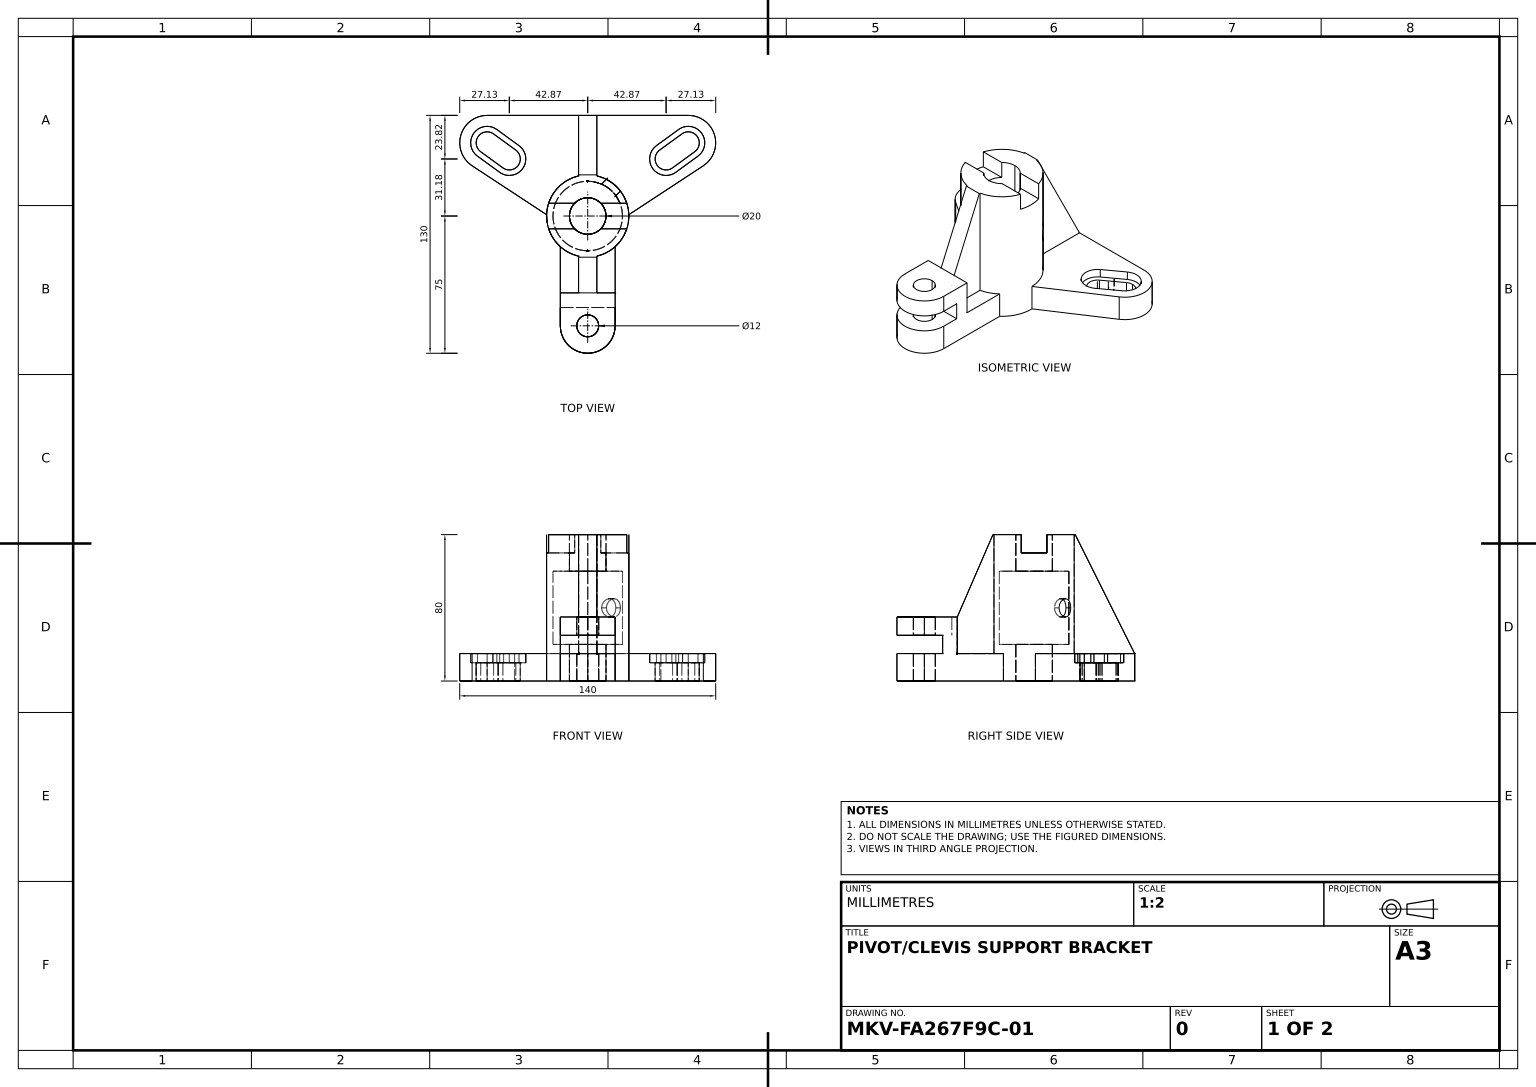
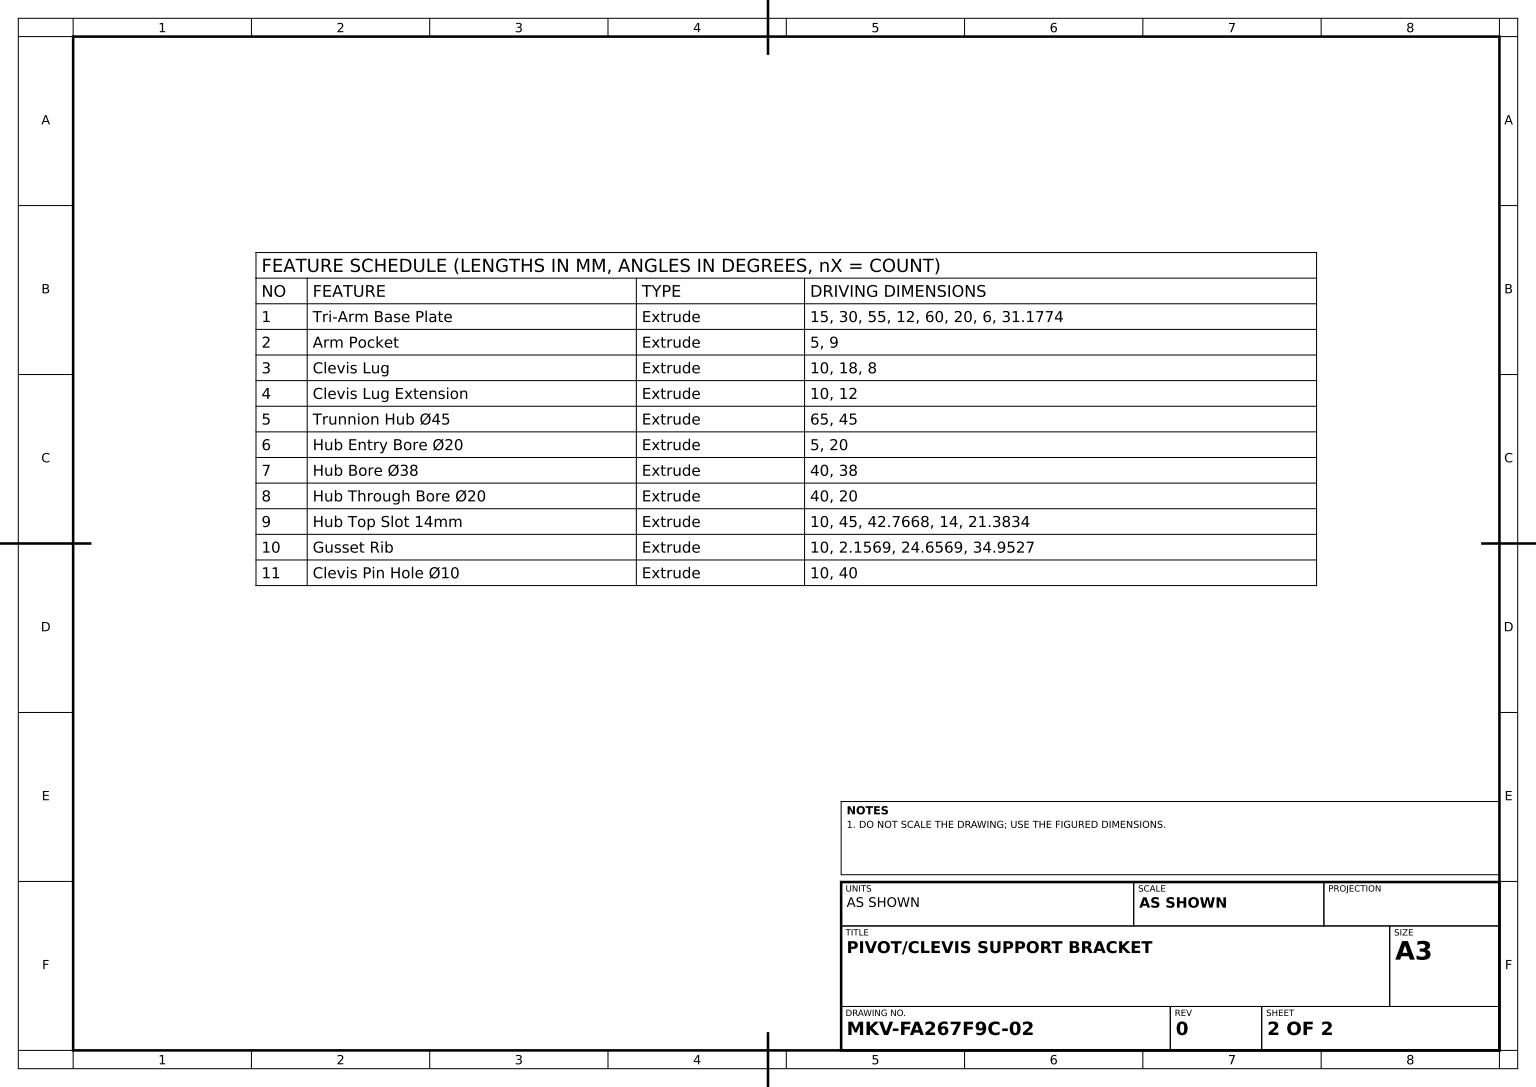
from build123d import *

# Parameters (mm, degrees)
TRI_ARM_BASE_PROFILE_R         = 22.5
TRI_ARM_BASE_PROFILE_R_2       = 10
TRI_ARM_BASE_PROFILE_R_3       = 6
TRI_ARM_BASE_PLATE_DEPTH       = 15
ARM_POCKET_DEPTH               = 5
CLEVIS_LUG_PROFILE_W           = 30
CLEVIS_LUG_PROFILE_H           = 8
CLEVIS_LUG_DEPTH               = 10
CLEVIS_LUG_EXTENSION_PROFILE_R = 6
CLEVIS_LUG_EXTENSION_DEPTH     = 10
TRUNNION_HUB_PROFILE_45_R      = 22.5
TRUNNION_HUB_45_DEPTH          = 65
HUB_ENTRY_BORE_PROFILE_20_R    = 10
HUB_ENTRY_BORE_20_DEPTH        = 5
HUB_BORE_PROFILE_38_R          = 19
HUB_BORE_38_DEPTH              = 40
HUB_START                      = -40
HUB_THROUGH_BORE_PROFILE_20_R  = 10
HUB_THROUGH_BORE_20_DEPTH      = 40
HUB_START_2                    = -10
HUB_TOP_SLOT_14MM_DEPTH        = 10
GUSSET_RIB_DEPTH               = 5
CLEVIS_PIN_HOLE_PROFILE_10_R   = 5
CLEVIS_PIN_HOLE_10_DEPTH       = 131.096118313


with BuildPart() as part:
    # Tri-Arm Base Profile → Tri-Arm Base Plate (new body)
    # profile 1 of 3: a face of its own
    with BuildSketch(Plane(origin=(0, 0, 0), x_dir=(1, 0, 0), z_dir=(0, 1, 0))):
        with BuildLine():
            Line((55, 55), (-55, 55))
            ThreePointArc((-55, 55), (-69.372088771, 44.294538898), (-63.22953257, 27.459075246))
            Line((-63.22953257, 27.459075246), (-22.488344437, 0.724130156))
            ThreePointArc((-22.488344437, 0.724130156), (0, 22.5), (22.488344437, 0.724130156))
            Line((22.488344437, 0.724130156), (63.22953257, 27.459075246))
            ThreePointArc((63.22953257, 27.459075246), (69.372088771, 44.294538898), (55, 55))
        make_face()
        with BuildLine():
            ThreePointArc((-58.529030186, 35.147583494), (-59.852416506, 43.529030186), (-51.470969814, 44.852416506))
            Line((-51.470969814, 44.852416506), (-39.339928549, 36.029841041))
            ThreePointArc((-39.339928549, 36.029841041), (-38.01654223, 27.648394349), (-46.397988922, 26.325008029))
            Line((-46.397988922, 26.325008029), (-58.529030186, 35.147583494))
        make_face(mode=Mode.SUBTRACT)
        with BuildLine():
            ThreePointArc((51.470969814, 44.852416506), (59.852416506, 43.529030186), (58.529030186, 35.147583494))
            Line((58.529030186, 35.147583494), (46.397988922, 26.325008029))
            ThreePointArc((46.397988922, 26.325008029), (38.01654223, 27.648394349), (39.339928549, 36.029841041))
            Line((39.339928549, 36.029841041), (51.470969814, 44.852416506))
        make_face(mode=Mode.SUBTRACT)
    # profile 2 of 3: a face of its own
    with BuildSketch(Plane(origin=(0, 0, 0), x_dir=(1, 0, 0), z_dir=(0, 1, 0))):
        Circle(TRI_ARM_BASE_PROFILE_R)
        with Locations(Location((0, 0, 0), (0, 0, 270))):
            Circle(TRI_ARM_BASE_PROFILE_R_2, mode=Mode.SUBTRACT)
    # profile 3 of 3: a face of its own
    with BuildSketch(Plane(origin=(0, 0, 0), x_dir=(1, 0, 0), z_dir=(0, 1, 0))):
        with BuildLine():
            ThreePointArc((15, -16.770509831), (0, -22.5), (-15, -16.770509831))
            Line((-15, -16.770509831), (-15, -60))
            ThreePointArc((-15, -60), (0, -75), (15, -60))
            Line((15, -60), (15, -16.770509831))
        make_face()
        with Locations(Location((0, -60, 0), (0, 0, 270))):
            Circle(TRI_ARM_BASE_PROFILE_R_3, mode=Mode.SUBTRACT)
    extrude(amount=TRI_ARM_BASE_PLATE_DEPTH)

    # Arm Pocket Profile → Arm Pocket (cut)
    with BuildSketch(Plane(origin=(0, 15, 0), x_dir=(1, 0, 0), z_dir=(0, 1, 0))):
        with BuildLine():
            Line((-49.706454721, 47.278624759), (-37.575413456, 38.456049294))
            ThreePointArc((-37.575413456, 38.456049294), (-35.590333977, 25.883879256), (-48.162504015, 23.898799776))
            Line((-48.162504015, 23.898799776), (-60.293545279, 32.721375241))
            ThreePointArc((-60.293545279, 32.721375241), (-62.278624759, 45.293545279), (-49.706454721, 47.278624759))
        make_face()
        with BuildLine():
            Line((37.575413456, 38.456049294), (49.706454721, 47.278624759))
            ThreePointArc((49.706454721, 47.278624759), (62.278624759, 45.293545279), (60.293545279, 32.721375241))
            Line((60.293545279, 32.721375241), (48.162504015, 23.898799776))
            ThreePointArc((48.162504015, 23.898799776), (35.590333977, 25.883879256), (37.575413456, 38.456049294))
        make_face()
    extrude(amount=-ARM_POCKET_DEPTH, mode=Mode.SUBTRACT)

    # Clevis Lug Profile → Clevis Lug (add)
    with BuildSketch(Plane(origin=(0, 15, 0), x_dir=(1, 0, 0), z_dir=(0, 1, 0))):
        with Locations((0, -46)):
            Rectangle(CLEVIS_LUG_PROFILE_W, CLEVIS_LUG_PROFILE_H)
    extrude(amount=CLEVIS_LUG_DEPTH)

    # Clevis Lug Extension Profile → Clevis Lug Extension (add)
    with BuildSketch(Plane(origin=(0, 25, 0), x_dir=(1, 0, 0), z_dir=(0, 1, 0))):
        with BuildLine():
            Line((-15, -42), (-15, -60))
            ThreePointArc((-15, -60), (0, -75), (15, -60))
            Line((15, -60), (15, -42))
            Line((15, -42), (-15, -42))
        make_face()
        with Locations(Location((0, -60, 0), (0, 0, 270))):
            Circle(CLEVIS_LUG_EXTENSION_PROFILE_R, mode=Mode.SUBTRACT)
    extrude(amount=CLEVIS_LUG_EXTENSION_DEPTH)

    # Trunnion Hub Profile Ø45 → Trunnion Hub Ø45 (add)
    with BuildSketch(Plane(origin=(0, 15, 0), x_dir=(1, 0, 0), z_dir=(0, 1, 0))):
        with Locations(Location((0, 0, 0), (0, 0, 1.844300776))):
            Circle(TRUNNION_HUB_PROFILE_45_R)
    extrude(amount=TRUNNION_HUB_45_DEPTH)

    # Hub Entry Bore Profile Ø20 → Hub Entry Bore Ø20 (cut)
    with BuildSketch(Plane.XZ.offset(-15)):
        with Locations(Location((0, 0, 0), (0, 0, 270))):
            Circle(HUB_ENTRY_BORE_PROFILE_20_R)
    extrude(amount=-HUB_ENTRY_BORE_20_DEPTH, mode=Mode.SUBTRACT)

    # Hub Bore Profile Ø38 → Hub Bore Ø38 (cut)
    with BuildSketch(Plane.XZ.offset(-20)):
        with Locations(Location((0, 0, 0), (0, 0, 270))):
            Circle(HUB_BORE_PROFILE_38_R)
    extrude(amount=-HUB_BORE_38_DEPTH, mode=Mode.SUBTRACT)

    # Hub Through Bore Profile Ø20 → Hub Through Bore Ø20 (cut)
    with BuildSketch(Plane(origin=(0, 80, 0), x_dir=(1, 0, 0), z_dir=(0, 1, 0)).offset(HUB_START)):
        with Locations(Location((0, 0, 0), (0, 0, 90))):
            Circle(HUB_THROUGH_BORE_PROFILE_20_R)
    extrude(amount=HUB_THROUGH_BORE_20_DEPTH, mode=Mode.SUBTRACT)

    # Hub Top Slot Profile → Hub Top Slot 14mm (cut)
    with BuildSketch(Plane(origin=(0, 80, 0), x_dir=(1, 0, 0), z_dir=(0, 1, 0)).offset(HUB_START_2)):
        with BuildLine():
            Line((-21.38340478, -7), (21.38340478, -7))
            ThreePointArc((21.38340478, -7), (22.5, 0), (21.38340478, 7))
            Line((21.38340478, 7), (-21.38340478, 7))
            ThreePointArc((-21.38340478, 7), (-22.5, 0), (-21.38340478, -7))
        make_face()
    extrude(amount=HUB_TOP_SLOT_14MM_DEPTH, mode=Mode.SUBTRACT)

    # Gusset Rib Profile → Gusset Rib (add, symmetric)
    with BuildSketch(Plane(origin=(0, 0, 0), x_dir=(0, 0, -1), z_dir=(1, 0, 0))):
        Polygon((-42, 35), (-22.5, 80), (-19.5, 80), (-19.5, 15), (-44.156903801, 15), (-44.156903801, 35), align=None)
        Polygon((22.5, 80), (55, 15), (20.047322275, 15), (20.047322275, 80), align=None)
    extrude(amount=GUSSET_RIB_DEPTH, both=True)

    # Clevis Pin Hole Profile Ø10 → Clevis Pin Hole Ø10 (cut, through all)
    with BuildSketch(Plane(origin=(0, 0, 0), x_dir=(0.7071067811865477, 0, 0.7071067811865475), z_dir=(-0.7071067811865475, 0, 0.7071067811865477))):
        with Locations((-1.976558152, 40)):
            Circle(CLEVIS_PIN_HOLE_PROFILE_10_R)
    extrude(amount=-CLEVIS_PIN_HOLE_10_DEPTH, mode=Mode.SUBTRACT)


solid = part.part
